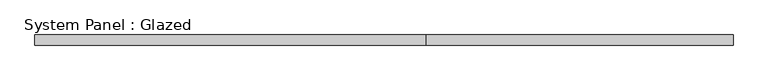
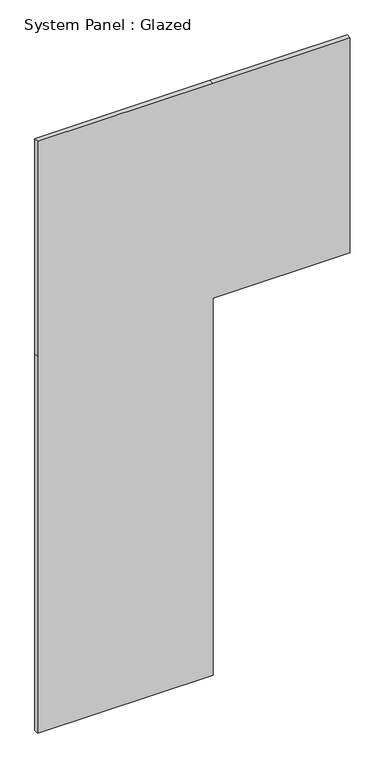
"""IFC4 building model written with IfcOpenShell, lengths in millimetres: plate geometry, System Panel : Glazed."""

from ifc_helpers import new_model, si_unit, frame, origin, place, context, project, spatial, polyline, outline, extrude, source, transform, mapped, element, save


def system_panel_glazed_ca5a80b0(model_context):
    return source(origin(), model_context, "Body", "SweptSolid", [
        extrude(outline(polyline([(0.0, -838.1560517), (0.0, 101.5560517), (2133.6, 101.5560517), (2133.6, 838.1560517), (3352.8, 838.1560517), (3352.8, 101.5560517), (3352.8, -838.1560517), (2133.6, -838.1560517), (0.0, -838.1560517)])), frame((0.0, 19.05, 0.0), z_axis=(0.0, 1.0, 0.0), x_axis=(0.0, 0.0, 1.0)), (0.0, 0.0, 1.0), 25.4),
    ])


if __name__ == "__main__":
    model = new_model("IFC4")
    model_context = context("Model", 3, world=origin())
    ifc_project = project(units=[si_unit("LENGTHUNIT", "METRE", prefix="MILLI")], contexts=[model_context])
    site = spatial("IfcSite", under=ifc_project)
    building = spatial("IfcBuilding", under=site)
    placement = place(None, origin())
    system_panel_glazed_shape = system_panel_glazed_ca5a80b0(model_context)
    element("IfcPlate", 1, ObjectType="System Panel : Glazed", at=placement, inside=building, context=model_context, shape_type="MappedRepresentation", body=[
        mapped(system_panel_glazed_shape, transform((0.0, 0.0, 0.0), x_axis=(1.0, 0.0, 0.0), y_axis=(0.0, 1.0, 0.0), z_axis=(0.0, 0.0, 1.0))),
    ])
    save(model, "model.ifc")

# Revit data of these elements
# Type "System Panel : Glazed"
#   Construction Type Id = "GSP4R"
#   Analytic Construction = "1/8 in Pilkington single glazing"
#   Visual Light Transmittance = 0.9
#   Solar Heat Gain Coefficient = 0.86
#   Heat Transfer Coefficient (U) = 1.18115 BTU/(h·ft²·°F)
#   Define Thermal Properties by = 1
# Element 1 (IfcPlate, "System Panel : Glazed")
#   Materials on its faces: "Glass"
# Materials
#   "Glass": class "Glass", colour RGB 0 128 192, transparency 0.75, Description = "Soda Lime Glass", Cost = 0
